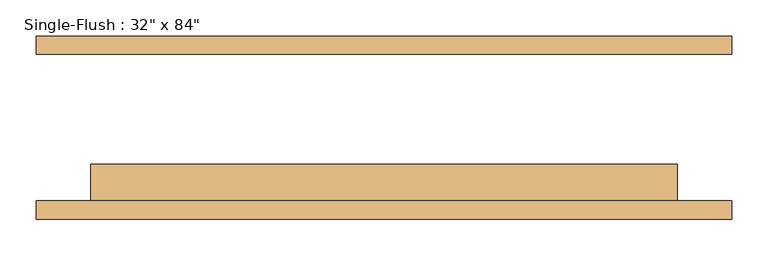
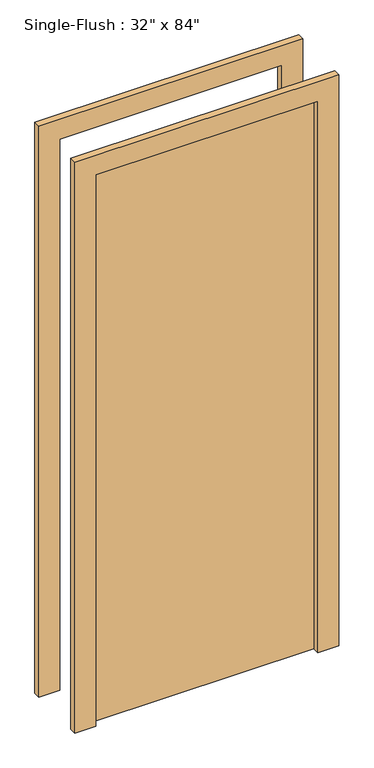
"""IFC4 building model written with IfcOpenShell, lengths in millimetres: door geometry."""

from ifc_helpers import new_model, si_unit, frame, origin, origin_with_axes, place, context, project, spatial, polyline, outline, extrude, source, transform, mapped, element, save


def door_0d629d65(model_context):
    return source(origin(), model_context, "Body", "SweptSolid", [
        extrude(outline(polyline([(2209.8, -482.6), (0.0, -482.6), (0.0, -406.4), (2133.6, -406.4), (2133.6, 406.4), (0.0, 406.4), (0.0, 482.6), (2209.8, 482.6), (2209.8, -482.6)])), frame((0.0, -127.0, 0.0), z_axis=(0.0, 1.0, 0.0), x_axis=(0.0, 0.0, 1.0)), (0.0, 0.0, 1.0), 25.4),
        extrude(outline(polyline([(2209.8, 482.6), (2209.8, -482.6), (0.0, -482.6), (0.0, -406.4), (2133.6, -406.4), (2133.6, 406.4), (0.0, 406.4), (0.0, 482.6), (2209.8, 482.6)])), frame((0.0, 101.6, 0.0), z_axis=(0.0, 1.0, 0.0), x_axis=(0.0, 0.0, 1.0)), (0.0, 0.0, 1.0), 25.4),
        extrude(outline(polyline([(406.4, -50.8), (406.4, -101.6), (-406.4, -101.6), (-406.4, -50.8), (406.4, -50.8)])), origin_with_axes(), (0.0, 0.0, 1.0), 2133.6),
    ])


if __name__ == "__main__":
    model = new_model("IFC4")
    model_context = context("Model", 3, world=origin())
    ifc_project = project(units=[si_unit("LENGTHUNIT", "METRE", prefix="MILLI")], contexts=[model_context])
    site = spatial("IfcSite", under=ifc_project)
    building = spatial("IfcBuilding", under=site)
    placement = place(None, origin())
    door_shape = door_0d629d65(model_context)
    element("IfcDoor", 1, ObjectType="Single-Flush : 32\" x 84\"", at=placement, inside=building, context=model_context, shape_type="MappedRepresentation", body=[
        mapped(door_shape, transform((0.0, 0.0, 0.0), x_axis=(1.0, 0.0, 0.0), y_axis=(0.0, 1.0, 0.0), z_axis=(0.0, 0.0, 1.0))),
    ])
    save(model, "model.ifc")

# Revit data of these elements
# Type "Single-Flush : 32\" x 84\""
#   Type Mark = "3"
#   Construction Type Id = "MDOOR"
#   Assembly Code = "C1020"
#   Analytic Construction = "Metal"
#   Thickness = 0' - 2"
#   Heat Transfer Coefficient (U) = 0.651978 BTU/(h·ft²·°F)
#   Height = 7' - 0"
#   Trim Projection Ext = 0' - 1"
#   Trim Projection Int = 0' - 1"
#   Trim Width = 0' - 3"
#   Width = 2' - 8"
#   Define Thermal Properties by = 1
#   Door Material = Door - Panel
#   Frame Material = Door - Frame
#   Visual Light Transmittance = 0
#   Solar Heat Gain Coefficient = 0
#   Function = (empty or 0)
#   Wall Closure = (empty or 0)
# Element 1 (IfcDoor, "Single-Flush : 32\" x 84\"")
#   Materials on its faces: "Door - Frame", "Door - Panel"
# Materials
#   "Door - Panel": class "Wood", colour RGB 210 159 95, transparency 0
#   "Door - Frame": colour RGB 118 70 51, transparency 0
